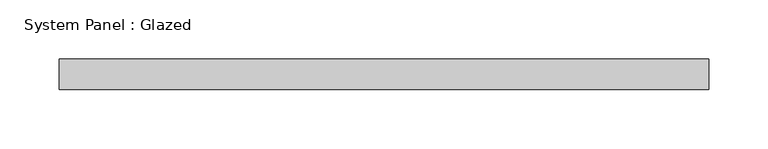
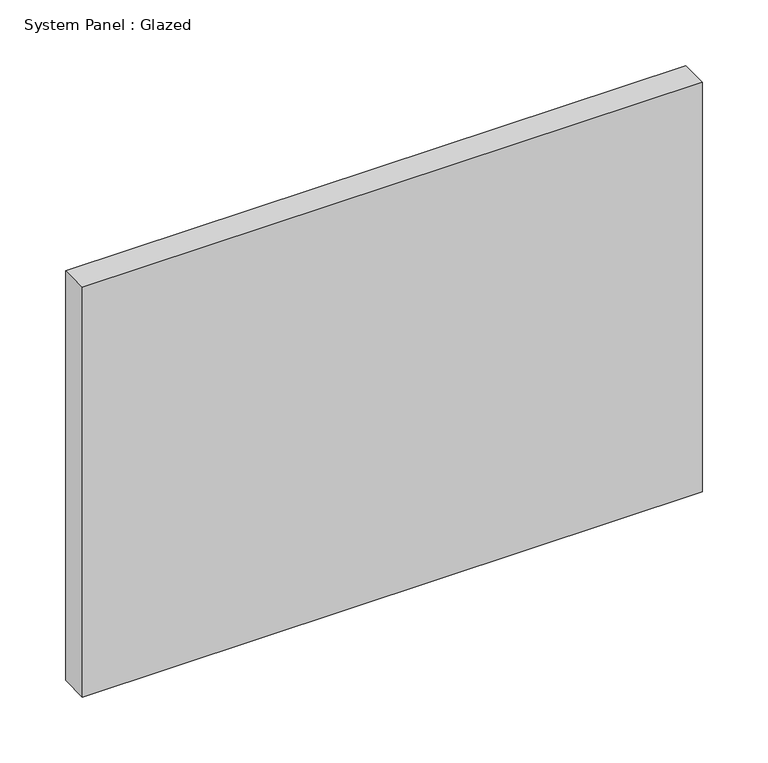
"""IFC4 building model written with IfcOpenShell, lengths in millimetres: plate geometry, System Panel : Glazed."""

from ifc_helpers import new_model, si_unit, origin, origin_with_axes, place, context, project, spatial, polyline, outline, extrude, source, transform, mapped, element, save


def system_panel_glazed_b66c72d1(model_context):
    return source(origin(), model_context, "Body", "SweptSolid", [
        extrude(outline(polyline([(273.05, 19.05), (-273.05, 19.05), (-273.05, 44.45), (273.05, 44.45), (273.05, 19.05)])), origin_with_axes(), (0.0, 0.0, 1.0), 381.2313568),
    ])


if __name__ == "__main__":
    model = new_model("IFC4")
    model_context = context("Model", 3, world=origin())
    ifc_project = project(units=[si_unit("LENGTHUNIT", "METRE", prefix="MILLI")], contexts=[model_context])
    site = spatial("IfcSite", under=ifc_project)
    building = spatial("IfcBuilding", under=site)
    placement = place(None, origin())
    system_panel_glazed_shape = system_panel_glazed_b66c72d1(model_context)
    element("IfcPlate", 1, ObjectType="System Panel : Glazed", at=placement, inside=building, context=model_context, shape_type="MappedRepresentation", body=[
        mapped(system_panel_glazed_shape, transform((0.0, 0.0, 0.0), x_axis=(1.0, 0.0, 0.0), y_axis=(0.0, 1.0, 0.0), z_axis=(0.0, 0.0, 1.0))),
    ])
    save(model, "model.ifc")

# Revit data of these elements
# Type "System Panel : Glazed"
#   Construction Type Id = "GSP4R"
#   Analytic Construction = "1/8 in Pilkington single glazing"
#   Visual Light Transmittance = 0.9
#   Solar Heat Gain Coefficient = 0.86
#   Heat Transfer Coefficient (U) = 1.18115 BTU/(h·ft²·°F)
#   Define Thermal Properties by = 1
# Element 1 (IfcPlate, "System Panel : Glazed")
#   Materials on its faces: "Glass"
# Materials
#   "Glass": class "Glass", colour RGB 0 128 192, transparency 0.75, Description = "Soda Lime Glass", Cost = 0
